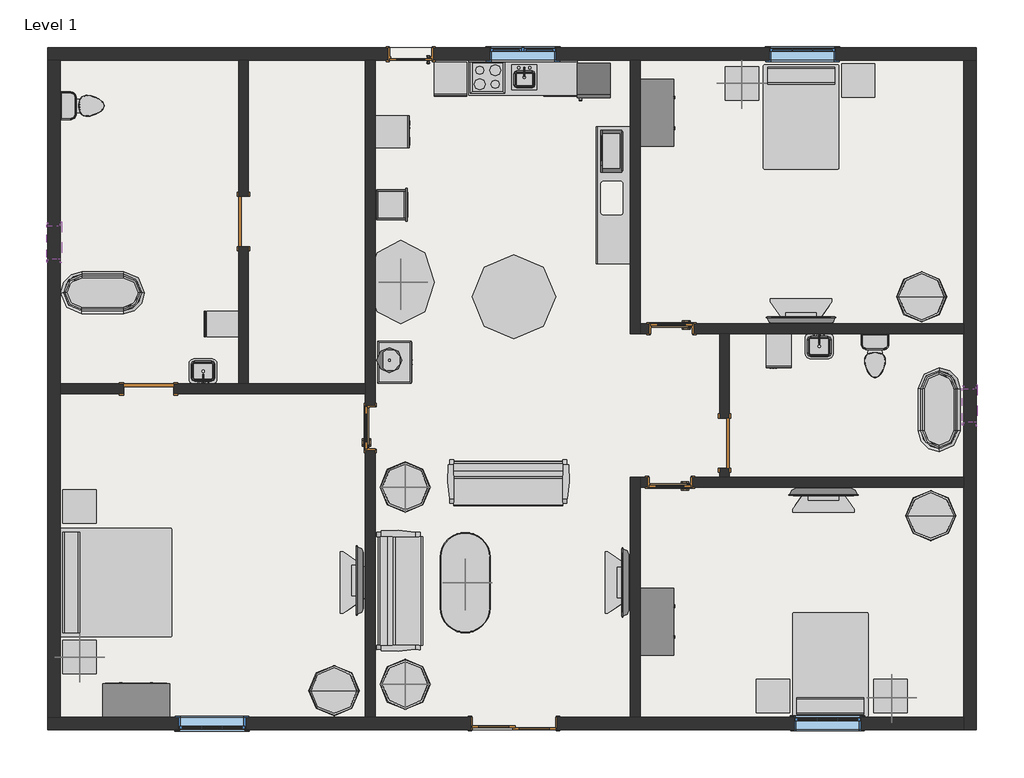
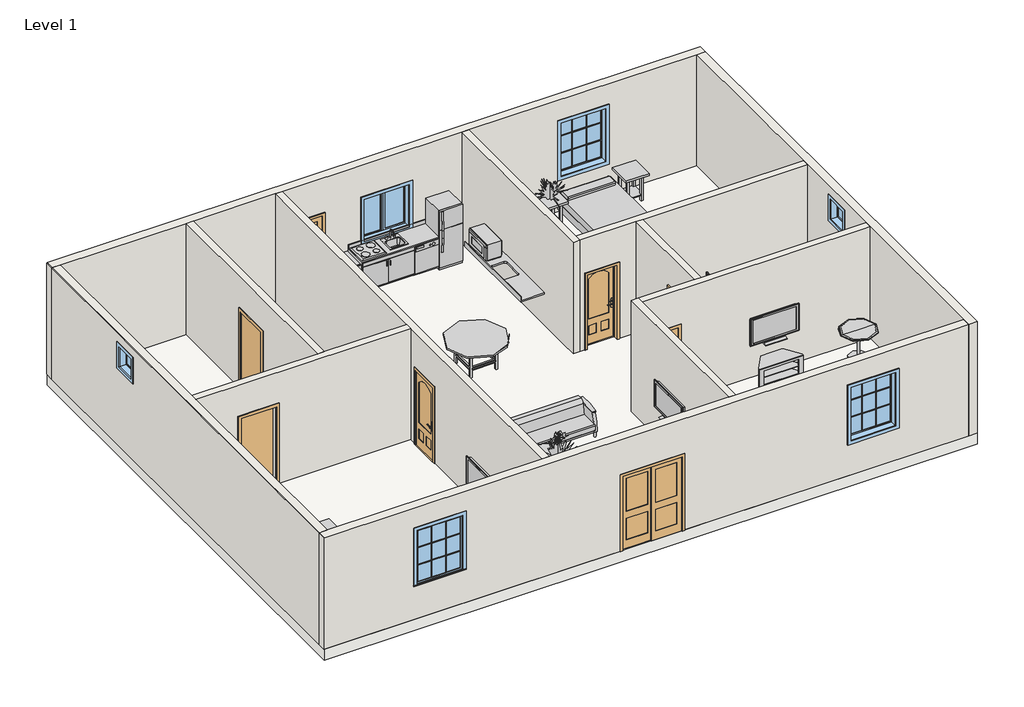
# One storey, incomplete: 33 furniture elements, 12 walls, 10 proxies, 8 doors, 8 flow terminals, 7 geographic elements, 6 windows, 1 slab.
"""IFC4 building model written with IfcOpenShell, lengths in millimetres."""

from ifc_helpers import new_model, si_unit, frame, origin, place, context, project, spatial, polyline, outline, extrude, faceted_brep, transform, mapped, element, save
from components import proxy_7e1014cc, proxy_a6faaae8, proxy_53e5fb40, proxy_45b28599, kitchenette_medium_kitchenette_medium_844211aa, proxy_8a8d5ab2, proxy_8b8c2dc4, proxy_c523a7b7, door_195c67e9, door_8a8e9806, door_61c74ce0, door_efd3daa1, door_90112511, flow_terminal_871c2e40, flow_terminal_d49f872f, flow_terminal_62a433f7, toilet_domestic_3d_toilet_domestic_3d_f7549cf7, toilet_domestic_3d_toilet_domestic_3d_183bbd19, flow_terminal_b374fae2, furniture_5bfe328f, furniture_0253826f, furniture_1fc5af50, counter_top_w_sink_hole_0600mm_depth_f226a61d, furniture_c6510c7c, furniture_9fa109b2, furniture_aff9b2fb, furniture_fdf74506, tv_stand_tv_stand_6ce107e5, furniture_2c34a4f9, furniture_bbcc68ce, furniture_743965d2, furniture_5bc9ed15, furniture_c80d6d9c, rpc_plant_tropical_55f6ff97, rpc_plant_tropical_agave_1_5_93a2a214, window_544f1267, window_d86b664e, window_534dcd48, window_3ed046d9

model = new_model("IFC4")

# Units and contexts
model_context = context("Model", 3, world=origin())
ifc_project = project(units=[si_unit("LENGTHUNIT", "METRE", prefix="MILLI")], contexts=[model_context])

# Site, building, storey
site = spatial("IfcSite", under=ifc_project)
building = spatial("IfcBuilding", under=site)
storey = spatial("IfcBuildingStorey", under=building, Name="Level 1", Elevation=0.0)

# Proxies
placement = place(None, origin())
proxy_shape = proxy_7e1014cc(model_context)
element("IfcBuildingElementProxy", 1, Name="18\" x 24\" x 34 1/2\"", ObjectType="18\" x 24\" x 34 1/2\"", at=placement, inside=storey, context=model_context, shape_type="MappedRepresentation", body=[
    mapped(proxy_shape, transform((-7798.9762552, 8109.3917392, 0.0), x_axis=(0.0, -1.0, 0.0), y_axis=(1.0, 0.0, 0.0), z_axis=(0.0, 0.0, 1.0))),
])
element("IfcBuildingElementProxy", 2, Name="18\" x 24\" x 34 1/2\"", ObjectType="18\" x 24\" x 34 1/2\"", at=placement, inside=storey, context=model_context, shape_type="MappedRepresentation", body=[
    mapped(proxy_shape, transform((2308.6558411, 7054.224706, 0.0), x_axis=(1.0, 0.0, 0.0), y_axis=(0.0, 1.0, 0.0), z_axis=(0.0, 0.0, 1.0))),
])
proxy_2_shape = proxy_a6faaae8(model_context)
element("IfcBuildingElementProxy", 3, Name="Cook Top-4 Unit2 : 22\" x 20\"", ObjectType="Cook Top-4 Unit2 : 22\" x 20\"", at=placement, inside=storey, context=model_context, shape_type="MappedRepresentation", body=[
    mapped(proxy_2_shape, transform((-2693.8266904, 12299.0742707, 0.0), x_axis=(1.0, 0.0, 0.0), y_axis=(0.0, 1.0, 0.0), z_axis=(0.0, 0.0, 1.0))),
])
proxy_3_shape = proxy_53e5fb40(model_context)
element("IfcBuildingElementProxy", 4, Name="Dishwasher : 23\" x 23 11/16\" x 33 1/2\"", ObjectType="Dishwasher : 23\" x 23 11/16\" x 33 1/2\"", at=placement, inside=storey, context=model_context, shape_type="MappedRepresentation", body=[
    mapped(proxy_3_shape, transform((-4167.2771257, 10932.5068022, 0.0), x_axis=(0.0, 1.0000000000000002, 0.0), y_axis=(-1.0000000000000002, 0.0, 0.0), z_axis=(0.0, 0.0, 1.0))),
])
element("IfcBuildingElementProxy", 5, Name="Dishwasher : 23\" x 23 11/16\" x 33 1/2\"", ObjectType="Dishwasher : 23\" x 23 11/16\" x 33 1/2\"", at=placement, inside=storey, context=model_context, shape_type="MappedRepresentation", body=[
    mapped(proxy_3_shape, transform((-3736.5441589, 12007.224706, 0.0), x_axis=(1.0, 0.0, 0.0), y_axis=(0.0, 1.0, 0.0), z_axis=(0.0, 0.0, 1.0))),
])
proxy_4_shape = proxy_45b28599(model_context)
element("IfcBuildingElementProxy", 6, Name="Dishwasher : 24\" x 24\" x 34\"", ObjectType="Dishwasher : 24\" x 24\" x 34\"", at=placement, inside=storey, context=model_context, shape_type="MappedRepresentation", body=[
    mapped(proxy_4_shape, transform((-1742.6441589, 12007.224706, 0.0), x_axis=(1.0, 0.0, 0.0), y_axis=(0.0, 1.0, 0.0), z_axis=(0.0, 0.0, 1.0))),
])
kitchenette_medium_kitchenette_medium_shape = kitchenette_medium_kitchenette_medium_844211aa(model_context)
element("IfcBuildingElementProxy", 7, Name="Kitchenette - Medium : Kitchenette - Medium", ObjectType="Kitchenette - Medium : Kitchenette - Medium", at=placement, inside=storey, context=model_context, shape_type="MappedRepresentation", body=[
    mapped(kitchenette_medium_kitchenette_medium_shape, transform((-2369.6643954, 12603.8742707, 0.0), x_axis=(1.0, 0.0, 0.0), y_axis=(0.0, 1.0, 0.0), z_axis=(0.0, 0.0, 1.0))),
])
proxy_5_shape = proxy_8a8d5ab2(model_context)
element("IfcBuildingElementProxy", 8, Name="Microwave : 30\" x 16\" x 18\"", ObjectType="Microwave : 30\" x 16\" x 18\"", at=placement, inside=storey, context=model_context, shape_type="MappedRepresentation", body=[
    mapped(proxy_5_shape, transform((-74.5899346, 11453.1671481, 0.0), x_axis=(0.0, -1.0000000000000004, 0.0), y_axis=(1.0000000000000004, 0.0, 0.0), z_axis=(0.0, 0.0, 1.0))),
])
proxy_6_shape = proxy_8b8c2dc4(model_context)
element("IfcBuildingElementProxy", 9, Name="Oven Double-Built-in : 21 1/2\" x 39 1/4\" x 21\"", ObjectType="Oven Double-Built-in : 21 1/2\" x 39 1/4\" x 21\"", at=placement, inside=storey, context=model_context, shape_type="MappedRepresentation", body=[
    mapped(proxy_6_shape, transform((-4305.3608315, 10010.149198, 0.0), x_axis=(0.0, 1.0000000000000002, 0.0), y_axis=(-1.0000000000000002, 0.0, 0.0), z_axis=(0.0, 0.0, 1.0))),
])
proxy_7_shape = proxy_c523a7b7(model_context)
element("IfcBuildingElementProxy", 10, Name="Refrigerator : 24\" x 25\" LH", ObjectType="Refrigerator : 24\" x 25\" LH", at=placement, inside=storey, context=model_context, shape_type="MappedRepresentation", body=[
    mapped(proxy_7_shape, transform((-757.0766904, 12253.4252993, 0.0), x_axis=(1.0, 0.0, 0.0), y_axis=(0.0, 1.0, 0.0), z_axis=(0.0, 0.0, 1.0))),
])

# Doors
door_shape = door_195c67e9(model_context)
element("IfcDoor", 11, ObjectType="30\" x 80\"", at=placement, inside=storey, context=model_context, shape_type="MappedRepresentation", body=[
    mapped(door_shape, transform((633.5733096, 4917.1992707, 0.0), x_axis=(1.0, 0.0, 0.0), y_axis=(0.0, 1.0, 0.0), z_axis=(0.0, 0.0, 1.0))),
])
element("IfcDoor", 12, ObjectType="30\" x 80\"", at=placement, inside=storey, context=model_context, shape_type="MappedRepresentation", body=[
    mapped(door_shape, transform((-4830.6016904, 5910.9742707, 0.0), x_axis=(0.0, -1.0, 0.0), y_axis=(1.0, 0.0, 0.0), z_axis=(0.0, 0.0, 1.0))),
])
door_2_shape = door_8a8e9806(model_context)
element("IfcDoor", 13, ObjectType="30\" x 80\"", at=placement, inside=storey, context=model_context, shape_type="MappedRepresentation", body=[
    mapped(door_2_shape, transform((658.9733096, 7717.5492707, 0.0), x_axis=(1.0, 0.0, 0.0), y_axis=(0.0, 1.0, 0.0), z_axis=(0.0, 0.0, 1.0))),
])
door_3_shape = door_61c74ce0(model_context)
element("IfcDoor", 14, ObjectType="Door-Interior-Double-Sliding-2_Panel-Wood : 60\" x 80\"", at=placement, inside=storey, context=model_context, shape_type="MappedRepresentation", body=[
    mapped(door_3_shape, transform((-2211.2266904, 522.9992707, 0.0), x_axis=(-1.0, 0.0, 0.0), y_axis=(0.0, -1.0, 0.0), z_axis=(0.0, 0.0, 1.0))),
])
door_4_shape = door_efd3daa1(model_context)
element("IfcDoor", 15, ObjectType="Door-Interior-Single-Full Glass-Wood : 30\" x 80\"", at=placement, inside=storey, context=model_context, shape_type="MappedRepresentation", body=[
    mapped(door_4_shape, transform((-4090.8266904, 12714.9992707, 0.0), x_axis=(-1.0, 0.0, 0.0), y_axis=(0.0, -1.0, 0.0), z_axis=(0.0, 0.0, 1.0))),
])
door_5_shape = door_90112511(model_context)
element("IfcDoor", 16, ObjectType="Single-Flush : 36\" x 84\"", at=placement, inside=storey, context=model_context, shape_type="MappedRepresentation", body=[
    mapped(door_5_shape, transform((-8866.0266904, 6622.1742707, 0.0), x_axis=(1.0, 0.0, 0.0), y_axis=(0.0, 1.0, 0.0), z_axis=(0.0, 0.0, 1.0))),
])
element("IfcDoor", 17, ObjectType="Single-Flush : 36\" x 84\"", at=placement, inside=storey, context=model_context, shape_type="MappedRepresentation", body=[
    mapped(door_5_shape, transform((-7138.8266904, 9670.1742707, 0.0), x_axis=(0.0, 1.0, 0.0), y_axis=(-1.0, 0.0, 0.0), z_axis=(0.0, 0.0, 1.0))),
])
element("IfcDoor", 18, ObjectType="Single-Flush : 36\" x 84\"", at=placement, inside=storey, context=model_context, shape_type="MappedRepresentation", body=[
    mapped(door_5_shape, transform((1624.1733096, 5631.5742707, 0.0), x_axis=(0.0, -1.0, 0.0), y_axis=(1.0, 0.0, 0.0), z_axis=(0.0, 0.0, 1.0))),
])

# Flow terminals
flow_terminal_shape = flow_terminal_871c2e40(model_context)
element("IfcFlowTerminal", 19, ObjectType="Sink Kitchen-Island : 18\" x 18\"", at=placement, inside=storey, context=model_context, shape_type="MappedRepresentation", body=[
    mapped(flow_terminal_shape, transform((-2036.415931, 12296.7288696, -14.4), x_axis=(1.0, 0.0, 0.0), y_axis=(0.0, 1.0, 0.0), z_axis=(0.0, 0.0, 1.0))),
])
flow_terminal_2_shape = flow_terminal_d49f872f(model_context)
element("IfcFlowTerminal", 20, ObjectType="Sink Vanity-Round : 19\" x 19\"", at=placement, inside=storey, context=model_context, shape_type="MappedRepresentation", body=[
    mapped(flow_terminal_2_shape, transform((-4396.1276023, 7046.2225302, 457.2), x_axis=(0.0, 1.0000000000000002, 0.0), y_axis=(-1.0000000000000002, 0.0, 0.0), z_axis=(0.0, 0.0, 1.0))),
])
flow_terminal_3_shape = flow_terminal_62a433f7(model_context)
element("IfcFlowTerminal", 21, ObjectType="Sink Vanity-Square : 20\" x 18\"", at=placement, inside=storey, context=model_context, shape_type="MappedRepresentation", body=[
    mapped(flow_terminal_3_shape, transform((-7859.7374499, 6891.2196719, 0.0), x_axis=(-1.0000000000000004, 0.0, 0.0), y_axis=(0.0, -1.0000000000000004, 0.0), z_axis=(0.0, 0.0, 1.0))),
])
element("IfcFlowTerminal", 22, ObjectType="Sink Vanity-Square : 20\" x 18\"", at=placement, inside=storey, context=model_context, shape_type="MappedRepresentation", body=[
    mapped(flow_terminal_3_shape, transform((3335.684069, 7445.3288696, 0.0), x_axis=(1.0, 0.0, 0.0), y_axis=(0.0, 1.0, 0.0), z_axis=(0.0, 0.0, 1.0))),
])
toilet_domestic_3d_toilet_domestic_3d_shape = toilet_domestic_3d_toilet_domestic_3d_f7549cf7(model_context)
toilet_domestic_3d_toilet_domestic_3d_2_shape = toilet_domestic_3d_toilet_domestic_3d_183bbd19(model_context)
element("IfcFlowTerminal", 23, ObjectType="Toilet-Domestic-3D : Toilet-Domestic-3D", at=placement, inside=storey, context=model_context, shape_type="MappedRepresentation", body=[
    mapped(toilet_domestic_3d_toilet_domestic_3d_shape, transform((-9984.2306631, 11778.3742707, 0.0), x_axis=(0.0, 1.0000000000000002, 0.0), y_axis=(-1.0000000000000002, 0.0, 0.0), z_axis=(0.0, 0.0, 1.0))),
    mapped(toilet_domestic_3d_toilet_domestic_3d_2_shape, transform((-9984.2306631, 11778.3742707, 0.0), x_axis=(0.0, 1.0000000000000002, 0.0), y_axis=(-1.0000000000000002, 0.0, 0.0), z_axis=(0.0, 0.0, 1.0))),
])
element("IfcFlowTerminal", 24, ObjectType="Toilet-Domestic-3D : Toilet-Domestic-3D", at=placement, inside=storey, context=model_context, shape_type="MappedRepresentation", body=[
    mapped(toilet_domestic_3d_toilet_domestic_3d_shape, transform((4367.3733096, 7130.7782434, 0.0), x_axis=(1.0, 0.0, 0.0), y_axis=(0.0, 1.0, 0.0), z_axis=(0.0, 0.0, 1.0))),
    mapped(toilet_domestic_3d_toilet_domestic_3d_2_shape, transform((4367.3733096, 7130.7782434, 0.0), x_axis=(1.0, 0.0, 0.0), y_axis=(0.0, 1.0, 0.0), z_axis=(0.0, 0.0, 1.0))),
])
flow_terminal_4_shape = flow_terminal_b374fae2(model_context)
element("IfcFlowTerminal", 25, ObjectType="Tub-Free Standing-3D : 30\" x 60\"", at=placement, inside=storey, context=model_context, shape_type="MappedRepresentation", body=[
    mapped(flow_terminal_4_shape, transform((-9704.2266904, 8374.7742707, 0.0), x_axis=(0.0, 1.0000000000000009, 0.0), y_axis=(-1.0000000000000009, 0.0, 0.0), z_axis=(0.0, 0.0, 1.0))),
])
element("IfcFlowTerminal", 26, ObjectType="Tub-Free Standing-3D : 30\" x 60\"", at=placement, inside=storey, context=model_context, shape_type="MappedRepresentation", body=[
    mapped(flow_terminal_4_shape, transform((5535.7733096, 6241.1742707, 0.0), x_axis=(1.0, 0.0, 0.0), y_axis=(0.0, 1.0, 0.0), z_axis=(0.0, 0.0, 1.0))),
])

# Furniture
furniture_shape = furniture_5bfe328f(model_context)
element("IfcFurniture", 27, ObjectType="Base Cabinet-Double Door Sink Unit : 30\"", at=placement, inside=storey, context=model_context, shape_type="MappedRepresentation", body=[
    mapped(furniture_shape, transform((-4694.0203208, 7086.0365658, 0.0), x_axis=(0.0, 1.0000000000000002, 0.0), y_axis=(-1.0000000000000002, 0.0, 0.0), z_axis=(0.0, 0.0, 1.0))),
])
furniture_2_shape = furniture_0253826f(model_context)
element("IfcFurniture", 28, ObjectType="Bed-Standard.0001 : Double 54\" x 75\"", at=placement, inside=storey, context=model_context, shape_type="MappedRepresentation", body=[
    mapped(furniture_2_shape, transform((2749.684785, 11620.7693527, 0.0), x_axis=(1.0, 0.0, 0.0), y_axis=(0.0, 1.0, 0.0), z_axis=(0.0, 0.0, 1.0))),
])
element("IfcFurniture", 29, ObjectType="Bed-Standard.0001 : Double 54\" x 75\"", at=placement, inside=storey, context=model_context, shape_type="MappedRepresentation", body=[
    mapped(furniture_2_shape, transform((3826.0618341, 1547.3791888, 0.0), x_axis=(-1.0000000000000004, 0.0, 0.0), y_axis=(0.0, -1.0000000000000004, 0.0), z_axis=(0.0, 0.0, 1.0))),
])
furniture_3_shape = furniture_1fc5af50(model_context)
element("IfcFurniture", 30, ObjectType="Bed-Standard.0001 : King 78\" x 80\"", at=placement, inside=storey, context=model_context, shape_type="MappedRepresentation", body=[
    mapped(furniture_3_shape, transform((-9508.5217724, 2820.0857461, 0.0), x_axis=(0.0, 1.0000000000000009, 0.0), y_axis=(-1.0000000000000009, 0.0, 0.0), z_axis=(0.0, 0.0, 1.0))),
])
counter_top_w_sink_hole_0600mm_depth_shape = counter_top_w_sink_hole_0600mm_depth_f226a61d(model_context)
element("IfcFurniture", 31, ObjectType="Counter Top w Sink Hole : 0600mm Depth", at=placement, inside=storey, context=model_context, shape_type="MappedRepresentation", body=[
    mapped(counter_top_w_sink_hole_0600mm_depth_shape, transform((-715.0079404, 10097.5240658, 0.0), x_axis=(0.0, 1.0000000000000002, 0.0), y_axis=(-1.0000000000000002, 0.0, 0.0), z_axis=(0.0, 0.0, 1.0))),
])
furniture_4_shape = furniture_c6510c7c(model_context)
element("IfcFurniture", 32, ObjectType="Counter Top w Sink Hole : 24\" Depth", at=placement, inside=storey, context=model_context, shape_type="MappedRepresentation", body=[
    mapped(furniture_4_shape, transform((-1836.2643954, 12603.8742707, -14.4), x_axis=(1.0, 0.0, 0.0), y_axis=(0.0, 1.0, 0.0), z_axis=(0.0, 0.0, 1.0))),
])
furniture_5_shape = furniture_9fa109b2(model_context)
element("IfcFurniture", 33, ObjectType="Dresser : 48\" x 72\" x 24\"", at=placement, inside=storey, context=model_context, shape_type="MappedRepresentation", body=[
    mapped(furniture_5_shape, transform((-9363.8199503, 582.1113166, 0.0), x_axis=(-1.0000000000000004, 0.0, 0.0), y_axis=(0.0, -1.0000000000000004, 0.0), z_axis=(0.0, 0.0, 1.0))),
])
element("IfcFurniture", 34, ObjectType="Dresser : 48\" x 72\" x 24\"", at=placement, inside=storey, context=model_context, shape_type="MappedRepresentation", body=[
    mapped(furniture_5_shape, transform((29.1103555, 11920.5675306, 0.0), x_axis=(0.0, 1.0000000000000002, 0.0), y_axis=(-1.0000000000000002, 0.0, 0.0), z_axis=(0.0, 0.0, 1.0))),
])
element("IfcFurniture", 35, ObjectType="Dresser : 48\" x 72\" x 24\"", at=placement, inside=storey, context=model_context, shape_type="MappedRepresentation", body=[
    mapped(furniture_5_shape, transform((29.1103555, 2649.5675306, 0.0), x_axis=(0.0, 1.0000000000000002, 0.0), y_axis=(-1.0000000000000002, 0.0, 0.0), z_axis=(0.0, 0.0, 1.0))),
])
furniture_6_shape = furniture_aff9b2fb(model_context)
element("IfcFurniture", 36, ObjectType="Sofa-Pensi : 84\"", at=placement, inside=storey, context=model_context, shape_type="MappedRepresentation", body=[
    mapped(furniture_6_shape, transform((-4016.9168544, 2660.5680207, 0.0), x_axis=(0.0, 1.0, 0.0), y_axis=(-1.0, 0.0, 0.0), z_axis=(0.0, 0.0, 1.0))),
])
element("IfcFurniture", 37, ObjectType="Sofa-Pensi : 84\"", at=placement, inside=storey, context=model_context, shape_type="MappedRepresentation", body=[
    mapped(furniture_6_shape, transform((-2591.4329404, 4630.5644347, 0.0), x_axis=(1.0000000000000002, 0.0, 0.0), y_axis=(0.0, 1.0000000000000002, 0.0), z_axis=(0.0, 0.0, 1.0))),
])
furniture_7_shape = furniture_fdf74506(model_context)
element("IfcFurniture", 38, ObjectType="TV - Flat Screen : 50\"", at=placement, inside=storey, context=model_context, shape_type="MappedRepresentation", body=[
    mapped(furniture_7_shape, transform((-5014.0724177, 3125.7297566, 495.3), x_axis=(0.0, -1.0, 0.0), y_axis=(1.0, 0.0, 0.0), z_axis=(0.0, 0.0, 1.0))),
])
element("IfcFurniture", 39, ObjectType="TV - Flat Screen : 50\"", at=placement, inside=storey, context=model_context, shape_type="MappedRepresentation", body=[
    mapped(furniture_7_shape, transform((3017.2287954, 7861.8128944, 495.3), x_axis=(-1.0, 0.0, 0.0), y_axis=(0.0, -1.0, 0.0), z_axis=(0.0, 0.0, 1.0))),
])
element("IfcFurniture", 40, ObjectType="TV - Flat Screen : 50\"", at=placement, inside=storey, context=model_context, shape_type="MappedRepresentation", body=[
    mapped(furniture_7_shape, transform((3431.5178237, 4747.5356471, 914.4), x_axis=(1.0, 0.0, 0.0), y_axis=(0.0, 1.0, 0.0), z_axis=(0.0, 0.0, 1.0))),
])
element("IfcFurniture", 41, ObjectType="TV - Flat Screen : 50\"", at=placement, inside=storey, context=model_context, shape_type="MappedRepresentation", body=[
    mapped(furniture_7_shape, transform((-174.2653141, 3087.6297566, 914.4), x_axis=(0.0, -1.0, 0.0), y_axis=(1.0, 0.0, 0.0), z_axis=(0.0, 0.0, 1.0))),
])
tv_stand_tv_stand_shape = tv_stand_tv_stand_6ce107e5(model_context)
element("IfcFurniture", 42, ObjectType="TV Stand : TV Stand", at=placement, inside=storey, context=model_context, shape_type="MappedRepresentation", body=[
    mapped(tv_stand_tv_stand_shape, transform((-4916.3266904, 3216.7622728, 0.0), x_axis=(0.0, -1.0, 0.0), y_axis=(1.0, 0.0, 0.0), z_axis=(0.0, 0.0, 1.0))),
])
element("IfcFurniture", 43, ObjectType="TV Stand : TV Stand", at=placement, inside=storey, context=model_context, shape_type="MappedRepresentation", body=[
    mapped(tv_stand_tv_stand_shape, transform((3146.3613116, 7803.2742707, 0.0), x_axis=(-1.0000000000000004, 0.0, 0.0), y_axis=(0.0, -1.0000000000000004, 0.0), z_axis=(0.0, 0.0, 1.0))),
])
element("IfcFurniture", 44, ObjectType="TV Stand : TV Stand", at=placement, inside=storey, context=model_context, shape_type="MappedRepresentation", body=[
    mapped(tv_stand_tv_stand_shape, transform((3302.3853075, 4831.4742707, 0.0), x_axis=(1.0, 0.0, 0.0), y_axis=(0.0, 1.0, 0.0), z_axis=(0.0, 0.0, 1.0))),
])
element("IfcFurniture", 45, ObjectType="TV Stand : TV Stand", at=placement, inside=storey, context=model_context, shape_type="MappedRepresentation", body=[
    mapped(tv_stand_tv_stand_shape, transform((-90.3266904, 3216.7622728, 0.0), x_axis=(0.0, -1.0, 0.0), y_axis=(1.0, 0.0, 0.0), z_axis=(0.0, 0.0, 1.0))),
])
furniture_8_shape = furniture_2c34a4f9(model_context)
element("IfcFurniture", 46, ObjectType="Table-Dining Oval : 36\" x 72\"", at=placement, inside=storey, context=model_context, shape_type="MappedRepresentation", body=[
    mapped(furniture_8_shape, transform((-3458.3250511, 3493.3939429, 0.0), x_axis=(0.0, 1.0, 0.0), y_axis=(-1.0, 0.0, 0.0), z_axis=(0.0, 0.0, 1.0))),
])
furniture_9_shape = furniture_bbcc68ce(model_context)
element("IfcFurniture", 47, ObjectType="Table-Dining Round w Chairs : 60\" Diameter", at=placement, inside=storey, context=model_context, shape_type="MappedRepresentation", body=[
    mapped(furniture_9_shape, transform((-2314.9086577, 8483.4529593, 0.0), x_axis=(1.0, 0.0, 0.0), y_axis=(0.0, 1.0, 0.0), z_axis=(0.0, 0.0, 1.0))),
])
furniture_10_shape = furniture_743965d2(model_context)
element("IfcFurniture", 48, ObjectType="Table-Ellipse : 60\" x 48\"", at=placement, inside=storey, context=model_context, shape_type="MappedRepresentation", body=[
    mapped(furniture_10_shape, transform((-4268.6266904, 8565.437297, 0.0), x_axis=(0.0, 1.0, 0.0), y_axis=(-1.0, 0.0, 0.0), z_axis=(0.0, 0.0, 1.0))),
])
furniture_11_shape = furniture_5bc9ed15(model_context)
element("IfcFurniture", 49, ObjectType="Table-Night Stand : 24\" x 24\" x 30\"", at=placement, inside=storey, context=model_context, shape_type="MappedRepresentation", body=[
    mapped(furniture_11_shape, transform((-10431.8603207, 1427.8742707, 0.0), x_axis=(1.0, 0.0, 0.0), y_axis=(0.0, 1.0, 0.0), z_axis=(0.0, 0.0, 1.0))),
])
element("IfcFurniture", 50, ObjectType="Table-Night Stand : 24\" x 24\" x 30\"", at=placement, inside=storey, context=model_context, shape_type="MappedRepresentation", body=[
    mapped(furniture_11_shape, transform((-10431.8603207, 4171.0742707, 0.0), x_axis=(1.0, 0.0, 0.0), y_axis=(0.0, 1.0, 0.0), z_axis=(0.0, 0.0, 1.0))),
])
element("IfcFurniture", 51, ObjectType="Table-Night Stand : 24\" x 24\" x 30\"", at=placement, inside=storey, context=model_context, shape_type="MappedRepresentation", body=[
    mapped(furniture_11_shape, transform((1633.1396793, 11879.9742707, 0.0), x_axis=(1.0, 0.0, 0.0), y_axis=(0.0, 1.0, 0.0), z_axis=(0.0, 0.0, 1.0))),
])
element("IfcFurniture", 52, ObjectType="Table-Night Stand : 24\" x 24\" x 30\"", at=placement, inside=storey, context=model_context, shape_type="MappedRepresentation", body=[
    mapped(furniture_11_shape, transform((3754.0396793, 11930.7742707, 0.0), x_axis=(1.0, 0.0, 0.0), y_axis=(0.0, 1.0, 0.0), z_axis=(0.0, 0.0, 1.0))),
])
element("IfcFurniture", 53, ObjectType="Table-Night Stand : 24\" x 24\" x 30\"", at=placement, inside=storey, context=model_context, shape_type="MappedRepresentation", body=[
    mapped(furniture_11_shape, transform((4338.2396793, 716.6742707, 0.0), x_axis=(1.0, 0.0, 0.0), y_axis=(0.0, 1.0, 0.0), z_axis=(0.0, 0.0, 1.0))),
])
element("IfcFurniture", 54, ObjectType="Table-Night Stand : 24\" x 24\" x 30\"", at=placement, inside=storey, context=model_context, shape_type="MappedRepresentation", body=[
    mapped(furniture_11_shape, transform((2204.6396793, 716.6742707, 0.0), x_axis=(1.0, 0.0, 0.0), y_axis=(0.0, 1.0, 0.0), z_axis=(0.0, 0.0, 1.0))),
])
furniture_12_shape = furniture_c80d6d9c(model_context)
element("IfcFurniture", 55, ObjectType="Table-Round : 36\" Diameter", at=placement, inside=storey, context=model_context, shape_type="MappedRepresentation", body=[
    mapped(furniture_12_shape, transform((-5487.8266904, 1123.0742707, 0.0), x_axis=(1.0, 0.0, 0.0), y_axis=(0.0, 1.0, 0.0), z_axis=(0.0, 0.0, 1.0))),
])
element("IfcFurniture", 56, ObjectType="Table-Round : 36\" Diameter", at=placement, inside=storey, context=model_context, shape_type="MappedRepresentation", body=[
    mapped(furniture_12_shape, transform((5218.2733096, 8298.5742707, 0.0), x_axis=(1.0, 0.0, 0.0), y_axis=(0.0, 1.0, 0.0), z_axis=(0.0, 0.0, 1.0))),
])
element("IfcFurniture", 57, ObjectType="Table-Round : 36\" Diameter", at=placement, inside=storey, context=model_context, shape_type="MappedRepresentation", body=[
    mapped(furniture_12_shape, transform((5383.3733096, 4310.7742707, 0.0), x_axis=(1.0, 0.0, 0.0), y_axis=(0.0, 1.0, 0.0), z_axis=(0.0, 0.0, 1.0))),
])
element("IfcFurniture", 58, ObjectType="Table-Round : 36\" Diameter", at=placement, inside=storey, context=model_context, shape_type="MappedRepresentation", body=[
    mapped(furniture_12_shape, transform((-4192.4266904, 1237.3742707, 0.0), x_axis=(1.0, 0.0, 0.0), y_axis=(0.0, 1.0, 0.0), z_axis=(0.0, 0.0, 1.0))),
])
element("IfcFurniture", 59, ObjectType="Table-Round : 36\" Diameter", at=placement, inside=storey, context=model_context, shape_type="MappedRepresentation", body=[
    mapped(furniture_12_shape, transform((-4192.4266904, 4831.4742707, 0.0), x_axis=(1.0, 0.0, 0.0), y_axis=(0.0, 1.0, 0.0), z_axis=(0.0, 0.0, 1.0))),
])

# Geographic elements
rpc_plant_tropical_shape = rpc_plant_tropical_55f6ff97(model_context)
element("IfcGeographicElement", 60, ObjectType="RPC Plant - Tropical", at=placement, inside=storey, context=model_context, shape_type="MappedRepresentation", body=[
    mapped(rpc_plant_tropical_shape, transform((-3100.2266904, 3091.5742707, 762.0), x_axis=(1.0, 0.0, 0.0), y_axis=(0.0, 1.0, 0.0), z_axis=(0.0, 0.0, 1.0))),
])
element("IfcGeographicElement", 61, ObjectType="RPC Plant - Tropical", at=placement, inside=storey, context=model_context, shape_type="MappedRepresentation", body=[
    mapped(rpc_plant_tropical_shape, transform((-4268.6266904, 8565.2742707, 762.0), x_axis=(1.0, 0.0, 0.0), y_axis=(0.0, 1.0, 0.0), z_axis=(0.0, 0.0, 1.0))),
])
rpc_plant_tropical_agave_1_5_shape = rpc_plant_tropical_agave_1_5_93a2a214(model_context)
element("IfcGeographicElement", 62, ObjectType="RPC Plant - Tropical : Agave - 1.5'", at=placement, inside=storey, context=model_context, shape_type="MappedRepresentation", body=[
    mapped(rpc_plant_tropical_agave_1_5_shape, transform((-4192.4266904, 4831.4742707, 762.0), x_axis=(1.0, 0.0, 0.0), y_axis=(0.0, 1.0, 0.0), z_axis=(0.0, 0.0, 1.0))),
])
element("IfcGeographicElement", 63, ObjectType="RPC Plant - Tropical : Agave - 1.5'", at=placement, inside=storey, context=model_context, shape_type="MappedRepresentation", body=[
    mapped(rpc_plant_tropical_agave_1_5_shape, transform((-4192.4266904, 1237.3742707, 762.0), x_axis=(1.0, 0.0, 0.0), y_axis=(0.0, 1.0, 0.0), z_axis=(0.0, 0.0, 1.0))),
])
element("IfcGeographicElement", 64, ObjectType="RPC Plant - Tropical : Agave - 1.5'", at=placement, inside=storey, context=model_context, shape_type="MappedRepresentation", body=[
    mapped(rpc_plant_tropical_agave_1_5_shape, transform((-10123.3266904, 1732.6742707, 762.0), x_axis=(1.0, 0.0, 0.0), y_axis=(0.0, 1.0, 0.0), z_axis=(0.0, 0.0, 1.0))),
])
element("IfcGeographicElement", 65, ObjectType="RPC Plant - Tropical : Agave - 1.5'", at=placement, inside=storey, context=model_context, shape_type="MappedRepresentation", body=[
    mapped(rpc_plant_tropical_agave_1_5_shape, transform((1941.6733096, 12184.7742707, 762.0), x_axis=(1.0, 0.0, 0.0), y_axis=(0.0, 1.0, 0.0), z_axis=(0.0, 0.0, 1.0))),
])
element("IfcGeographicElement", 66, ObjectType="RPC Plant - Tropical : Agave - 1.5'", at=placement, inside=storey, context=model_context, shape_type="MappedRepresentation", body=[
    mapped(rpc_plant_tropical_agave_1_5_shape, transform((4672.1733096, 996.0742707, 762.0), x_axis=(1.0, 0.0, 0.0), y_axis=(0.0, 1.0, 0.0), z_axis=(0.0, 0.0, 1.0))),
])

# Slab
element("IfcSlab", 67, ObjectType="Generic - 12\"", at=placement, inside=storey, context=model_context, shape_type="SweptSolid", body=[
    extrude(outline(polyline([(6208.8733096, 12832.4742707), (6208.8733096, 411.8742707), (-10694.8266904, 411.8742707), (-10694.8266904, 12832.4742707), (6208.8733096, 12832.4742707)])), frame((0.0, 0.0, -304.8), z_axis=(0.0, 0.0, 1.0), x_axis=(1.0, 0.0, 0.0)), (0.0, 0.0, 1.0), 304.8),
])

# Walls
element("IfcWall", 68, ObjectType="Generic - 8\"", at=placement, inside=storey, context=model_context, shape_type="Brep", body=[
    faceted_brep([(6208.8733096, 12603.8742707, 0.0), (6208.8733096, 12603.8742707, 3048.0), (5980.2733096, 12603.8742707, 3048.0), (87.4733096, 12603.8742707, 3048.0), (-90.3266904, 12603.8742707, 3048.0), (-4738.5266904, 12603.8742707, 3048.0), (-4916.3266904, 12603.8742707, 3048.0), (-7049.9266904, 12603.8742707, 3048.0), (-7227.7266904, 12603.8742707, 3048.0), (-10478.9266904, 12603.8742707, 3048.0), (-10694.8266904, 12603.8742707, 3048.0), (-10707.5266904, 12603.8742707, 3048.0), (-10707.5266904, 12603.8742707, 0.0), (-10478.9266904, 12603.8742707, 0.0), (-7227.7266904, 12603.8742707, 0.0), (-7049.9266904, 12603.8742707, 0.0), (-4916.3266904, 12603.8742707, 0.0), (-4738.5266904, 12603.8742707, 0.0), (-4497.2266904, 12603.8742707, 0.0), (-4497.2266904, 12603.8742707, 2057.4), (-3684.4266904, 12603.8742707, 2057.4), (-3684.4266904, 12603.8742707, 0.0), (-90.3266904, 12603.8742707, 0.0), (87.4733096, 12603.8742707, 0.0), (5980.2733096, 12603.8742707, 0.0), (3656.1733096, 12603.8742707, 2438.4), (3656.1733096, 12603.8742707, 914.4), (2436.9733096, 12603.8742707, 914.4), (2436.9733096, 12603.8742707, 2438.4), (-1436.5266904, 12603.8742707, 2133.6), (-1436.5266904, 12603.8742707, 914.4), (-2655.7266904, 12603.8742707, 914.4), (-2655.7266904, 12603.8742707, 2133.6), (6208.8733096, 12832.4742707, 3048.0), (6208.8733096, 12832.4742707, 0.0), (-3684.4266904, 12832.4742707, 0.0), (-3684.4266904, 12832.4742707, 2057.4), (-4497.2266904, 12832.4742707, 2057.4), (-4497.2266904, 12832.4742707, 0.0), (-10707.5266904, 12832.4742707, 0.0), (-10707.5266904, 12832.4742707, 3048.0), (-10694.8266904, 12832.4742707, 3048.0), (3656.1733096, 12832.4742707, 2438.4), (2436.9733096, 12832.4742707, 2438.4), (2436.9733096, 12832.4742707, 914.4), (3656.1733096, 12832.4742707, 914.4), (-1436.5266904, 12832.4742707, 2133.6), (-2655.7266904, 12832.4742707, 2133.6), (-2655.7266904, 12832.4742707, 914.4), (-1436.5266904, 12832.4742707, 914.4)], [[[0, 1, 2, 3, 4, 5, 6, 7, 8, 9, 10, 11, 12, 13, 14, 15, 16, 17, 18, 19, 20, 21, 22, 23, 24], [25, 26, 27, 28], [29, 30, 31, 32]], [[33, 34, 35, 36, 37, 38, 39, 40, 41], [42, 43, 44, 45], [46, 47, 48, 49]], [[34, 0, 24, 23, 22, 21, 35]], [[12, 39, 38, 18, 17, 16, 15, 14, 13]], [[1, 0, 34, 33]], [[12, 11, 40, 39]], [[37, 19, 18, 38]], [[19, 37, 36, 20]], [[20, 36, 35, 21]], [[26, 25, 42, 45]], [[27, 26, 45, 44]], [[28, 27, 44, 43]], [[25, 28, 43, 42]], [[30, 29, 46, 49]], [[31, 30, 49, 48]], [[32, 31, 48, 47]], [[29, 32, 47, 46]], [[40, 11, 10, 41]], [[10, 9, 8, 7, 6, 5, 4, 3, 2, 1, 33, 41]]]),
])
element("IfcWall", 69, ObjectType="Generic - 8\"", at=placement, inside=storey, context=model_context, shape_type="Brep", body=[
    faceted_brep([(5980.2733096, 12603.8742707, 0.0), (5980.2733096, 7803.2742707, 0.0), (5980.2733096, 7625.4742707, 0.0), (5980.2733096, 5009.2742707, 0.0), (5980.2733096, 4831.4742707, 0.0), (5980.2733096, 640.4742707, 0.0), (5980.2733096, 411.8742707, 0.0), (5980.2733096, 411.8742707, 3048.0), (5980.2733096, 640.4742707, 3048.0), (5980.2733096, 4831.4742707, 3048.0), (5980.2733096, 5009.2742707, 3048.0), (5980.2733096, 7625.4742707, 3048.0), (5980.2733096, 7803.2742707, 3048.0), (5980.2733096, 12603.8742707, 3048.0), (5980.2733096, 6012.5742707, 2768.6), (5980.2733096, 6012.5742707, 2159.0), (5980.2733096, 6622.1742707, 2159.0), (5980.2733096, 6622.1742707, 2768.6), (6208.8733096, 12603.8742707, 0.0), (6208.8733096, 12603.8742707, 3048.0), (6208.8733096, 411.8742707, 3048.0), (6208.8733096, 411.8742707, 0.0), (6208.8733096, 6012.5742707, 2768.6), (6208.8733096, 6622.1742707, 2768.6), (6208.8733096, 6622.1742707, 2159.0), (6208.8733096, 6012.5742707, 2159.0)], [[[0, 1, 2, 3, 4, 5, 6, 7, 8, 9, 10, 11, 12, 13], [14, 15, 16, 17]], [[18, 19, 20, 21], [22, 23, 24, 25]], [[6, 5, 4, 3, 2, 1, 0, 18, 21]], [[0, 13, 19, 18]], [[7, 6, 21, 20]], [[13, 12, 11, 10, 9, 8, 7, 20, 19]], [[15, 14, 22, 25]], [[16, 15, 25, 24]], [[17, 16, 24, 23]], [[14, 17, 23, 22]]]),
])
element("IfcWall", 70, ObjectType="Generic - 8\"", at=placement, inside=storey, context=model_context, shape_type="Brep", body=[
    faceted_brep([(5980.2733096, 640.4742707, 3048.0), (5980.2733096, 640.4742707, 0.0), (87.4733096, 640.4742707, 0.0), (-90.3266904, 640.4742707, 0.0), (-1423.8266904, 640.4742707, 0.0), (-1423.8266904, 640.4742707, 2057.4), (-2998.6266904, 640.4742707, 2057.4), (-2998.6266904, 640.4742707, 0.0), (-4738.5266904, 640.4742707, 0.0), (-4916.3266904, 640.4742707, 0.0), (-10478.9266904, 640.4742707, 0.0), (-10707.5266904, 640.4742707, 0.0), (-10707.5266904, 640.4742707, 3048.0), (-10694.8266904, 640.4742707, 3048.0), (-10478.9266904, 640.4742707, 3048.0), (-4916.3266904, 640.4742707, 3048.0), (-4738.5266904, 640.4742707, 3048.0), (-90.3266904, 640.4742707, 3048.0), (87.4733096, 640.4742707, 3048.0), (-8319.9266904, 640.4742707, 2438.4), (-8319.9266904, 640.4742707, 914.4), (-7100.7266904, 640.4742707, 914.4), (-7100.7266904, 640.4742707, 2438.4), (2894.1733096, 640.4742707, 2438.4), (2894.1733096, 640.4742707, 914.4), (4113.3733096, 640.4742707, 914.4), (4113.3733096, 640.4742707, 2438.4), (5980.2733096, 411.8742707, 0.0), (5980.2733096, 411.8742707, 3048.0), (-10694.8266904, 411.8742707, 3048.0), (-10707.5266904, 411.8742707, 3048.0), (-10707.5266904, 411.8742707, 0.0), (-2998.6266904, 411.8742707, 0.0), (-2998.6266904, 411.8742707, 2057.4), (-1423.8266904, 411.8742707, 2057.4), (-1423.8266904, 411.8742707, 0.0), (-8319.9266904, 411.8742707, 2438.4), (-7100.7266904, 411.8742707, 2438.4), (-7100.7266904, 411.8742707, 914.4), (-8319.9266904, 411.8742707, 914.4), (2894.1733096, 411.8742707, 2438.4), (4113.3733096, 411.8742707, 2438.4), (4113.3733096, 411.8742707, 914.4), (2894.1733096, 411.8742707, 914.4)], [[[0, 1, 2, 3, 4, 5, 6, 7, 8, 9, 10, 11, 12, 13, 14, 15, 16, 17, 18], [19, 20, 21, 22], [23, 24, 25, 26]], [[27, 28, 29, 30, 31, 32, 33, 34, 35], [36, 37, 38, 39], [40, 41, 42, 43]], [[1, 27, 35, 4, 3, 2]], [[31, 11, 10, 9, 8, 7, 32]], [[1, 0, 28, 27]], [[12, 11, 31, 30]], [[6, 33, 32, 7]], [[33, 6, 5, 34]], [[34, 5, 4, 35]], [[20, 19, 36, 39]], [[21, 20, 39, 38]], [[22, 21, 38, 37]], [[19, 22, 37, 36]], [[24, 23, 40, 43]], [[25, 24, 43, 42]], [[26, 25, 42, 41]], [[23, 26, 41, 40]], [[12, 30, 29, 13]], [[0, 18, 17, 16, 15, 14, 13, 29, 28]]]),
])
element("IfcWall", 71, ObjectType="Generic - 8\"", at=placement, inside=storey, context=model_context, shape_type="Brep", body=[
    faceted_brep([(-10478.9266904, 640.4742707, 0.0), (-10478.9266904, 6533.2742707, 0.0), (-10478.9266904, 6711.0742707, 0.0), (-10478.9266904, 12603.8742707, 0.0), (-10478.9266904, 12603.8742707, 3048.0), (-10478.9266904, 6711.0742707, 3048.0), (-10478.9266904, 6533.2742707, 3048.0), (-10478.9266904, 640.4742707, 3048.0), (-10478.9266904, 8984.3742707, 2768.6), (-10478.9266904, 9593.9742707, 2768.6), (-10478.9266904, 9593.9742707, 2159.0), (-10478.9266904, 8984.3742707, 2159.0), (-10707.5266904, 640.4742707, 0.0), (-10707.5266904, 640.4742707, 3048.0), (-10707.5266904, 12603.8742707, 3048.0), (-10707.5266904, 12603.8742707, 0.0), (-10707.5266904, 8984.3742707, 2768.6), (-10707.5266904, 8984.3742707, 2159.0), (-10707.5266904, 9593.9742707, 2159.0), (-10707.5266904, 9593.9742707, 2768.6), (-10694.8266904, 12603.8742707, 3048.0), (-10694.8266904, 640.4742707, 3048.0)], [[[0, 1, 2, 3, 4, 5, 6, 7], [8, 9, 10, 11]], [[12, 13, 14, 15], [16, 17, 18, 19]], [[3, 2, 1, 0, 12, 15]], [[4, 3, 15, 14, 20]], [[0, 7, 21, 13, 12]], [[20, 14, 13, 21]], [[7, 6, 5, 4, 20, 21]], [[17, 16, 8, 11]], [[18, 17, 11, 10]], [[19, 18, 10, 9]], [[16, 19, 9, 8]]]),
])
element("IfcWall", 72, ObjectType="INNER WALLS", at=placement, inside=storey, context=model_context, shape_type="Brep", body=[
    faceted_brep([(-4916.3266904, 12603.8742707, 3048.0), (-4916.3266904, 12603.8742707, 0.0), (-4916.3266904, 6711.0742707, 0.0), (-4916.3266904, 6533.2742707, 0.0), (-4916.3266904, 6317.3742707, 0.0), (-4916.3266904, 6317.3742707, 2057.4), (-4916.3266904, 5504.5742707, 2057.4), (-4916.3266904, 5504.5742707, 0.0), (-4916.3266904, 640.4742707, 0.0), (-4916.3266904, 640.4742707, 3048.0), (-4916.3266904, 6533.2742707, 3048.0), (-4916.3266904, 6711.0742707, 3048.0), (-4738.5266904, 12603.8742707, 0.0), (-4738.5266904, 12603.8742707, 3048.0), (-4738.5266904, 640.4742707, 3048.0), (-4738.5266904, 640.4742707, 0.0), (-4738.5266904, 5504.5742707, 0.0), (-4738.5266904, 5504.5742707, 2057.4), (-4738.5266904, 6317.3742707, 2057.4), (-4738.5266904, 6317.3742707, 0.0)], [[[0, 1, 2, 3, 4, 5, 6, 7, 8, 9, 10, 11]], [[12, 13, 14, 15, 16, 17, 18, 19]], [[1, 12, 19, 4, 3, 2]], [[15, 8, 7, 16]], [[1, 0, 13, 12]], [[9, 8, 15, 14]], [[6, 17, 16, 7]], [[17, 6, 5, 18]], [[18, 5, 4, 19]], [[0, 11, 10, 9, 14, 13]]]),
])
element("IfcWall", 73, ObjectType="INNER WALLS", at=placement, inside=storey, context=model_context, shape_type="Brep", body=[
    faceted_brep([(-8408.8266904, 6533.2742707, 2133.6), (-8408.8266904, 6533.2742707, 0.0), (-4916.3266904, 6533.2742707, 0.0), (-4916.3266904, 6533.2742707, 3048.0), (-10478.9266904, 6533.2742707, 3048.0), (-10478.9266904, 6533.2742707, 0.0), (-9323.2266904, 6533.2742707, 0.0), (-9323.2266904, 6533.2742707, 2133.6), (-4916.3266904, 6711.0742707, 0.0), (-7049.9266904, 6711.0742707, 0.0), (-7227.7266904, 6711.0742707, 0.0), (-8408.8266904, 6711.0742707, 0.0), (-8408.8266904, 6711.0742707, 2133.6), (-9323.2266904, 6711.0742707, 2133.6), (-9323.2266904, 6711.0742707, 0.0), (-10478.9266904, 6711.0742707, 0.0), (-10478.9266904, 6711.0742707, 3048.0), (-7227.7266904, 6711.0742707, 3048.0), (-7049.9266904, 6711.0742707, 3048.0), (-4916.3266904, 6711.0742707, 3048.0)], [[[0, 1, 2, 3, 4, 5, 6, 7]], [[8, 9, 10, 11, 12, 13, 14, 15, 16, 17, 18, 19]], [[6, 5, 15, 14]], [[2, 1, 11, 10, 9, 8]], [[5, 4, 16, 15]], [[3, 2, 8, 19]], [[12, 11, 1, 0]], [[13, 12, 0, 7]], [[14, 13, 7, 6]], [[4, 3, 19, 18, 17, 16]]]),
])
element("IfcWall", 74, ObjectType="INNER WALLS", at=placement, inside=storey, context=model_context, shape_type="SweptSolid", body=[
    extrude(outline(polyline([(12603.8742707, 0.0), (10127.3742707, 0.0), (10127.3742707, 2133.6), (9212.9742707, 2133.6), (9212.9742707, 0.0), (6711.0742707, 0.0), (6711.0742707, 3048.0), (12603.8742707, 3048.0), (12603.8742707, 0.0)])), frame((-7227.7266904, 0.0, 0.0), z_axis=(1.0, 0.0, 0.0), x_axis=(0.0, 1.0, 0.0)), (0.0, 0.0, 1.0), 177.8),
])
element("IfcWall", 75, ObjectType="INNER WALLS", at=placement, inside=storey, context=model_context, shape_type="Brep", body=[
    faceted_brep([(-90.3266904, 12603.8742707, 0.0), (-90.3266904, 7625.4742707, 0.0), (-90.3266904, 7625.4742707, 3048.0), (-90.3266904, 12603.8742707, 3048.0), (87.4733096, 12603.8742707, 0.0), (87.4733096, 12603.8742707, 3048.0), (87.4733096, 7803.2742707, 3048.0), (87.4733096, 7625.4742707, 3048.0), (87.4733096, 7625.4742707, 0.0), (87.4733096, 7803.2742707, 0.0)], [[[0, 1, 2, 3]], [[4, 5, 6, 7, 8, 9]], [[1, 0, 4, 9, 8]], [[0, 3, 5, 4]], [[2, 1, 8, 7]], [[3, 2, 7, 6, 5]]]),
])
element("IfcWall", 76, ObjectType="INNER WALLS", at=placement, inside=storey, context=model_context, shape_type="Brep", body=[
    faceted_brep([(5980.2733096, 7803.2742707, 3048.0), (5980.2733096, 7803.2742707, 0.0), (1065.3733096, 7803.2742707, 0.0), (1065.3733096, 7803.2742707, 2057.4), (252.5733096, 7803.2742707, 2057.4), (252.5733096, 7803.2742707, 0.0), (87.4733096, 7803.2742707, 0.0), (87.4733096, 7803.2742707, 3048.0), (5980.2733096, 7625.4742707, 0.0), (5980.2733096, 7625.4742707, 3048.0), (1713.0733096, 7625.4742707, 3048.0), (1535.2733096, 7625.4742707, 3048.0), (87.4733096, 7625.4742707, 3048.0), (87.4733096, 7625.4742707, 0.0), (252.5733096, 7625.4742707, 0.0), (252.5733096, 7625.4742707, 2057.4), (1065.3733096, 7625.4742707, 2057.4), (1065.3733096, 7625.4742707, 0.0), (1535.2733096, 7625.4742707, 0.0), (1713.0733096, 7625.4742707, 0.0)], [[[0, 1, 2, 3, 4, 5, 6, 7]], [[8, 9, 10, 11, 12, 13, 14, 15, 16, 17, 18, 19]], [[1, 8, 19, 18, 17, 2]], [[13, 6, 5, 14]], [[1, 0, 9, 8]], [[7, 6, 13, 12]], [[16, 3, 2, 17]], [[3, 16, 15, 4]], [[4, 15, 14, 5]], [[0, 7, 12, 11, 10, 9]]]),
])
element("IfcWall", 77, ObjectType="INNER WALLS", at=placement, inside=storey, context=model_context, shape_type="Brep", body=[
    faceted_brep([(5980.2733096, 5009.2742707, 3048.0), (5980.2733096, 5009.2742707, 0.0), (1713.0733096, 5009.2742707, 0.0), (1535.2733096, 5009.2742707, 0.0), (1039.9733096, 5009.2742707, 0.0), (1039.9733096, 5009.2742707, 2057.4), (227.1733096, 5009.2742707, 2057.4), (227.1733096, 5009.2742707, 0.0), (87.4733096, 5009.2742707, 0.0), (87.4733096, 5009.2742707, 3048.0), (1535.2733096, 5009.2742707, 3048.0), (1713.0733096, 5009.2742707, 3048.0), (5980.2733096, 4831.4742707, 0.0), (5980.2733096, 4831.4742707, 3048.0), (87.4733096, 4831.4742707, 3048.0), (87.4733096, 4831.4742707, 0.0), (227.1733096, 4831.4742707, 0.0), (227.1733096, 4831.4742707, 2057.4), (1039.9733096, 4831.4742707, 2057.4), (1039.9733096, 4831.4742707, 0.0)], [[[0, 1, 2, 3, 4, 5, 6, 7, 8, 9, 10, 11]], [[12, 13, 14, 15, 16, 17, 18, 19]], [[1, 12, 19, 4, 3, 2]], [[15, 8, 7, 16]], [[1, 0, 13, 12]], [[18, 5, 4, 19]], [[5, 18, 17, 6]], [[6, 17, 16, 7]], [[9, 8, 15, 14]], [[0, 11, 10, 9, 14, 13]]]),
])
element("IfcWall", 78, ObjectType="INNER WALLS", at=placement, inside=storey, context=model_context, shape_type="Brep", body=[
    faceted_brep([(-90.3266904, 5009.2742707, 0.0), (-90.3266904, 640.4742707, 0.0), (-90.3266904, 640.4742707, 3048.0), (-90.3266904, 5009.2742707, 3048.0), (87.4733096, 5009.2742707, 0.0), (87.4733096, 5009.2742707, 3048.0), (87.4733096, 4831.4742707, 3048.0), (87.4733096, 640.4742707, 3048.0), (87.4733096, 640.4742707, 0.0), (87.4733096, 4831.4742707, 0.0)], [[[0, 1, 2, 3]], [[4, 5, 6, 7, 8, 9]], [[1, 0, 4, 9, 8]], [[2, 1, 8, 7]], [[0, 3, 5, 4]], [[3, 2, 7, 6, 5]]]),
])
element("IfcWall", 79, ObjectType="INNER WALLS", at=placement, inside=storey, context=model_context, shape_type="SweptSolid", body=[
    extrude(outline(polyline([(5174.3742707, 2133.6), (5174.3742707, 0.0), (5009.2742707, 0.0), (5009.2742707, 3048.0), (7625.4742707, 3048.0), (7625.4742707, 0.0), (6088.7742707, 0.0), (6088.7742707, 2133.6), (5174.3742707, 2133.6)])), frame((1535.2733096, 0.0, 0.0), z_axis=(1.0, 0.0, 0.0), x_axis=(0.0, 1.0, 0.0)), (0.0, 0.0, 1.0), 177.8),
])

# Windows
window_shape = window_544f1267(model_context)
element("IfcWindow", 80, ObjectType="Casement 3x3 with Trim : 48\" x 60\"", at=placement, inside=storey, context=model_context, shape_type="MappedRepresentation", body=[
    mapped(window_shape, transform((-7710.3266904, 526.1742707, 609.6), x_axis=(-1.0, 0.0, 0.0), y_axis=(0.0, -1.0, 0.0), z_axis=(0.0, 0.0, 1.0))),
])
element("IfcWindow", 81, ObjectType="Casement 3x3 with Trim : 48\" x 60\"", at=placement, inside=storey, context=model_context, shape_type="MappedRepresentation", body=[
    mapped(window_shape, transform((3046.5733096, 12718.1742707, 609.6), x_axis=(1.0, 0.0, 0.0), y_axis=(0.0, 1.0, 0.0), z_axis=(0.0, 0.0, 1.0))),
])
window_2_shape = window_d86b664e(model_context)
element("IfcWindow", 82, ObjectType="Casement 3x3 with Trim : 48\" x 60\"", at=placement, inside=storey, context=model_context, shape_type="MappedRepresentation", body=[
    mapped(window_2_shape, transform((3503.7733096, 526.1742707, 609.6), x_axis=(-1.0, 0.0, 0.0), y_axis=(0.0, -1.0, 0.0), z_axis=(0.0, 0.0, 1.0))),
])
window_3_shape = window_534dcd48(model_context)
element("IfcWindow", 83, ObjectType="Casement Dbl with Trim : 48\" x 48\"", at=placement, inside=storey, context=model_context, shape_type="MappedRepresentation", body=[
    mapped(window_3_shape, transform((-2046.1266904, 12699.1242707, 0.0), x_axis=(1.0, 0.0, 0.0), y_axis=(0.0, 1.0, 0.0), z_axis=(0.0, 0.0, 1.0))),
])
window_4_shape = window_3ed046d9(model_context)
element("IfcWindow", 84, ObjectType="Transom with Trim : 24\" x 24\"", at=placement, inside=storey, context=model_context, shape_type="MappedRepresentation", body=[
    mapped(window_4_shape, transform((6094.5733096, 6279.2742707, 0.0), x_axis=(0.0, -1.0, 0.0), y_axis=(1.0, 0.0, 0.0), z_axis=(0.0, 0.0, 1.0))),
])
element("IfcWindow", 85, ObjectType="Transom with Trim : 24\" x 24\"", at=placement, inside=storey, context=model_context, shape_type="MappedRepresentation", body=[
    mapped(window_4_shape, transform((-10593.2266904, 9251.0742707, 0.0), x_axis=(0.0, -1.0, 0.0), y_axis=(1.0, 0.0, 0.0), z_axis=(0.0, 0.0, 1.0))),
])

save(model, "model.ifc")

# Revit data of these elements
# Type "18\" x 24\" x 34 1/2\""
#   Label = "T"
#   Assembly Code = "E1090400"
#   Depth = 2' - 0"
#   Height = 2' - 10 1/2"
#   Width = 1' - 6"
#   Panel Face Material = Plastic, Opaque Black
#   Trach Compact. Material = Steel, Paint Finish, Ivory, Matte
#   Default Elevation = 0
# Type "Cook Top-4 Unit2 : 22\" x 20\""
#   Depth = 1' - 8"
#   Width = 1' - 10"
#   Burner Material = Steel, Chrome Plated
#   Cooktop Material = Steel, Polished
#   Default Elevation = 0
#   Assembly Code = ""
# Type "Dishwasher : 23\" x 23 11/16\" x 33 1/2\""
#   Label = "DW"
#   Assembly Code = "E1090400"
#   Depth = 1' - 11 11/16"
#   Height = 2' - 9 1/2"
#   Width = 1' - 11"
#   Dishwasher Material = Steel, Paint Finish, Ivory, Glossy
#   Panel Face Material = Plastic, Opaque Black
#   Default Elevation = 0
# Type "Dishwasher : 24\" x 24\" x 34\""
#   Label = "DW"
#   Assembly Code = "E1090400"
#   Depth = 2' - 0"
#   Height = 2' - 10"
#   Width = 2' - 0"
#   Dishwasher Material = Steel, Paint Finish, Ivory, Glossy
#   Panel Face Material = Plastic, Opaque Black
#   Default Elevation = 0
# Type "Kitchenette - Medium : Kitchenette - Medium"
#   Assembly Code = "E1090400"
#   Counter Length = 6' - 6"
#   Cabinet Width = 4' - 6"
#   Cabinet Height = 2' - 10 1/2"
#   Cabinet Depth = 2' - 0"
#   Toe Depth = 0' - 3"
#   Toe Height = 0' - 3 1/2"
#   Cabinet Material = Cabinets
#   Door/Drawer Material = Cabinets
#   Handle Material = Cabinets - Handles
#   Default Elevation = 0
# Type "Microwave : 30\" x 16\" x 18\""
#   Assembly Code = "E1090400"
#   Depth = 1' - 4"
#   Height = 1' - 6"
#   Width = 2' - 6"
#   Microwave Material = Laminate, Ivory, Matte
#   Default Elevation = 0
# Type "Oven Double-Built-in : 21 1/2\" x 39 1/4\" x 21\""
#   Label = "OVEN"
#   Assembly Code = "E1090400"
#   Depth = 1' - 9"
#   Height = 3' - 3 1/4"
#   Width = 1' - 9 1/2"
#   Oven Material = Metal - Stainless Steel, Polished
#   Default Elevation = 0
# Type "Refrigerator : 24\" x 25\" LH"
#   Label = "REF."
#   Assembly Code = "E1090400"
#   Depth = 2' - 0 3/4"
#   Handle = 0' - 1 1/2"
#   Height = 5' - 3 1/2"
#   Rear Clearance = 0' - 2"
#   Top Door Height = 1' - 8"
#   Width = 1' - 11 1/2"
#   Material = Steel, Paint Finish, Ivory, Glossy
#   Default Elevation = 0
# Type "30\" x 80\""
#   Type Mark = "9"
#   Assembly Code = "B2030100"
#   Analytic Construction = "French door, wood frame with single glass"
#   Threshold Offset [instance default] = 0' - 0 1/2"
#   Thickness = 0' - 1 3/8"
#   Thermal Resistance (R) = 1.0696 (h·ft²·°F)/BTU
#   Swing Angle [instance default] = 90.00°
#   Stiles = 0' - 4 3/4"
#   Rough Width = 2' - 8"
#   Rough Height = 6' - 9"
#   Radius = 1' - 1.00625"
#   Lock Rail = 0' - 7 1/8"
#   Height = 6' - 8"
#   Width = 2' - 6"
#   Heat Transfer Coefficient (U) = 0.9350 BTU/(h·ft²·°F)
#   Door Offset [instance default] = 0' - 0"
#   Bottom Rail = 0' - 9 1/2"
#   Threshold [instance default] = yes
#   Function = 1
#   Exterior Trim [instance default] = yes
#   Trim Material = Cherry
#   Threshold Material = Cherry
#   Panel Material = Cherry
#   Glazing = Glass
#   Frame Material = Cherry
#   Door Handle Material = Aluminum
#   Visual Light Transmittance = 0
#   Solar Heat Gain Coefficient = 0
#   Wall Closure = (empty or 0)
#   Construction Type = (empty or 0)
# Type "Door-Interior-Double-Sliding-2_Panel-Wood : 60\" x 80\""
#   Type Mark = "8"
#   Assembly Code = "C1020300"
#   Analytic Construction = "Wooden"
#   Top Rail = 0' - 4 11/16"
#   Thickness = 0' - 1 3/8"
#   Thermal Resistance (R) = 2.5876 (h·ft²·°F)/BTU
#   Stiles = 0' - 4 3/4"
#   Rough Width = 5' - 2"
#   Rough Height = 6' - 9"
#   Lock Rail = 0' - 7 1/2"
#   Height = 6' - 8"
#   Width = 5' - 0"
#   Heat Transfer Coefficient (U) = 0.3865 BTU/(h·ft²·°F)
#   Bottom Rail = 0' - 9 1/8"
#   Trim Material = Cherry
#   Panel Material = Cherry
#   Frame Material = Cherry
#   Visual Light Transmittance = 0
#   Solar Heat Gain Coefficient = 0
#   Wall Closure = (empty or 0)
#   Function = (empty or 0)
# Type "Door-Interior-Single-Full Glass-Wood : 30\" x 80\""
#   Type Mark = "10"
#   Assembly Code = "C1020300"
#   Analytic Construction = "Wood frame with single clear glass"
#   Top Rail = 0' - 4 11/16"
#   Thickness = 0' - 1 3/8"
#   Thermal Resistance (R) = 1.0102 (h·ft²·°F)/BTU
#   Swing Angle [instance default] = 90.00°
#   Stiles = 0' - 4 3/4"
#   Rough Width = 2' - 8"
#   Rough Height = 6' - 9"
#   Height = 6' - 8"
#   Width = 2' - 6"
#   Heat Transfer Coefficient (U) = 0.9900 BTU/(h·ft²·°F)
#   Bottom Rail = 0' - 9 1/8"
#   Show Grill [instance default] = yes
#   Trim Material = Cherry
#   Panel Material = Cherry
#   Frame Material = Cherry
#   Door Handle Material = Aluminum
#   Visual Light Transmittance = 0
#   Solar Heat Gain Coefficient = 0
#   Wall Closure = (empty or 0)
#   Function = (empty or 0)
# Type "Single-Flush : 36\" x 84\""
#   Type Mark = "1"
#   Construction Type Id = "MDOOR"
#   Assembly Code = "C1020"
#   Analytic Construction = "Metal"
#   Thickness = 0' - 2"
#   Heat Transfer Coefficient (U) = 0.651978 BTU/(h·ft²·°F)
#   Height = 7' - 0"
#   Trim Projection Ext = 0' - 1"
#   Trim Projection Int = 0' - 1"
#   Trim Width = 0' - 3"
#   Width = 3' - 0"
#   Define Thermal Properties by = 1
#   Door Material = Door - Panel
#   Frame Material = Door - Frame
#   Visual Light Transmittance = 0
#   Solar Heat Gain Coefficient = 0
#   Function = (empty or 0)
#   Wall Closure = (empty or 0)
# Type "Sink Kitchen-Island : 18\" x 18\""
#   Assembly Code = "D2010410"
#   Counter Height = 3' - 0"
#   Depth = 1' - 6"
#   Width = 1' - 6"
#   Faucet Material = Steel, Polished
#   Sink Material = Steel, Polished
#   Default Elevation = 0
# Type "Sink Vanity-Round : 19\" x 19\""
#   Assembly Code = "D2010400"
#   Top Of Counter = 2' - 7"
#   Basin Material = Porcelain, Linen
#   Faucet Material = Steel, Polished
#   Default Elevation = 0
# Type "Sink Vanity-Square : 20\" x 18\""
#   Assembly Code = "D2010400"
#   Counter Height = 2' - 7"
#   Depth = 1' - 6"
#   Width = 1' - 8"
#   Basin Material = Porcelain, Linen
#   Faucet Material = Steel, Polished
#   Default Elevation = 0
# Type "Toilet-Domestic-3D : Toilet-Domestic-3D"
#   Assembly Code = "D2010110"
#   Toilet - Bowl/Basin Material = Porcelain, Linen
#   Toilet - Seat Material = Laminate, Linen, Matte
#   Default Elevation = 0
# Type "Tub-Free Standing-3D : 30\" x 60\""
#   Assembly Code = "D2010110"
#   Height = 1' - 6"
#   Length = 5' - 0"
#   Width = 2' - 6"
#   Tub Material = Porcelain, Ivory
#   Default Elevation = 0
# Type "Base Cabinet-Double Door Sink Unit : 30\""
#   Assembly Code = "C1030410"
#   Depth = 2' - 0"
#   Height = 2' - 10 1/2"
#   Toe Depth = 0' - 3"
#   Toe Height = 0' - 3 1/2"
#   Width = 2' - 6"
#   Cabinet Material = none
#   Door/Drawer Material = none
#   Handle Material = Cabinets - Handles
#   Default Elevation = 0
# Type "Bed-Standard.0001 : Double 54\" x 75\""
#   Assembly Code = "E2020200"
#   Length = 6' - 3"
#   Width = 4' - 6"
#   Leg Material = Steel, Chrome Plated
#   Mattress Material = Linen, White
#   Default Elevation = 0
# Type "Bed-Standard.0001 : King 78\" x 80\""
#   Assembly Code = "E2020200"
#   Length = 6' - 8"
#   Width = 6' - 6"
#   Leg Material = Steel, Chrome Plated
#   Mattress Material = Linen, White
#   Default Elevation = 0
# Type "Counter Top w Sink Hole : 0600mm Depth"
#   Assembly Code = "C1030400"
#   Counter Thickness = 0' - 1 9/16"
#   Depth = 2' - 0 19/32"
#   Height = 2' - 11 7/16"
#   Length [instance default] = 8' - 2 7/16"
#   Sink Location [instance default] = 3' - 11 1/4"
#   Sink Location To Wall [instance default] = 0' - 3 15/16"
#   Sink Opening Depth [instance default] = 1' - 2 7/8"
#   Sink Opening Width [instance default] = 1' - 11 1/8"
#   Counter Top Material = none
#   Default Elevation = 0
# Type "Counter Top w Sink Hole : 24\" Depth"
#   Assembly Code = "C1030400"
#   Counter Thickness = 0' - 1 1/2"
#   Depth = 2' - 1"
#   Height = 3' - 0"
#   Length [instance default] = 8' - 0"
#   Sink Location [instance default] = 2' - 0"
#   Sink Location To Wall [instance default] = 0' - 6"
#   Sink Opening Depth [instance default] = 1' - 3"
#   Sink Opening Width [instance default] = 2' - 3"
#   Counter Top Material = none
#   Default Elevation = 0
# Type "Dresser : 48\" x 72\" x 24\""
#   Assembly Code = "E2020200"
#   Depth = 2' - 0"
#   Height = 6' - 0"
#   Width = 4' - 0"
#   Dresser Material = Laminate - Ivory, Glossy
#   Drawer Material = Laminate, Ivory, Matte
#   Knob Material = Cherry
#   Default Elevation = 0
# Type "Sofa-Pensi : 84\""
#   Assembly Code = "E2020200"
#   Length = 7' - 0"
#   Frame Material = Cherry
#   Seat Material = Linen, Beige
#   Feet Material = Steel, Chrome Plated
#   Default Elevation = 0
# Type "TV - Flat Screen : 50\""
#   SinAng = 0' - 0.0193"
#   L = 3' - 7.57782"
#   H = 2' - 0.51477"
#   Thickness = 0' - 4.33071"
#   Diagonal = 4' - 2"
#   CosAng = 0' - 0.03431"
#   Stand [instance default] = yes
#   Default Elevation = 0
# Type "TV Stand : TV Stand"
#   Depth = 1' - 6"
#   Width = 3' - 8"
#   Height = 1' - 7 1/2"
#   Finish = Melamine - Gray
#   Default Elevation = 0
# Type "Table-Dining Oval : 36\" x 72\""
#   Assembly Code = "E2020200"
#   Length = 6' - 0"
#   Width = 3' - 0"
#   Base Material = Steel, Chrome Plated
#   Top Material = Glass - Clear, Grey
#   Default Elevation = 0
#   Description = (empty or 0)
# Type "Table-Dining Round w Chairs : 60\" Diameter"
